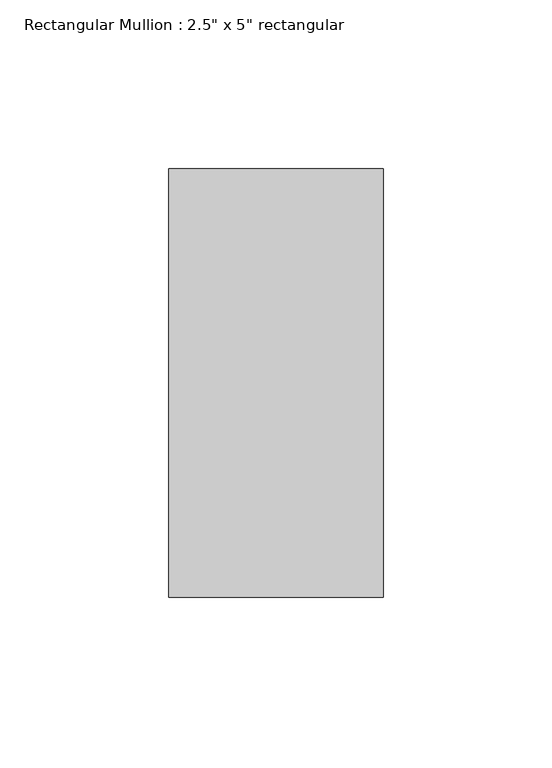
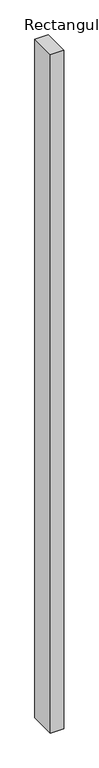
"""IFC4 building model written with IfcOpenShell, lengths in millimetres: member geometry."""

from ifc_helpers import new_model, si_unit, frame, origin, place, context, project, spatial, polyline, outline, extrude, source, transform, mapped, element, save


def member_6024fe87(model_context):
    return source(origin(), model_context, "Body", "SweptSolid", [
        extrude(outline(polyline([(0.0, 63.5), (0.0, -63.5), (-63.5, -63.5), (-63.5, 63.5), (0.0, 63.5)])), frame((0.0, 0.0, -3383.9874947), z_axis=(0.0, 0.0, 1.0), x_axis=(1.0, 0.0, 0.0)), (0.0, 0.0, 1.0), 3383.9874947),
    ])


if __name__ == "__main__":
    model = new_model("IFC4")
    model_context = context("Model", 3, world=origin())
    ifc_project = project(units=[si_unit("LENGTHUNIT", "METRE", prefix="MILLI")], contexts=[model_context])
    site = spatial("IfcSite", under=ifc_project)
    building = spatial("IfcBuilding", under=site)
    placement = place(None, origin())
    member_shape = member_6024fe87(model_context)
    element("IfcMember", 1, ObjectType="Rectangular Mullion : 2.5\" x 5\" rectangular", at=placement, inside=building, context=model_context, shape_type="MappedRepresentation", body=[
        mapped(member_shape, transform((0.0, 0.0, 0.0), x_axis=(1.0, 0.0, 0.0), y_axis=(0.0, 1.0, 0.0), z_axis=(0.0, 0.0, 1.0))),
    ])
    save(model, "model.ifc")

# Revit data of these elements
# Type "Rectangular Mullion : 2.5\" x 5\" rectangular"
#   built-in parameter 1007304 = 0.416667 (stored number, unit not read)
#   built-in parameter 1007301 = 0.104167 (stored number, unit not read)
#   built-in parameter 1007300 = 0.104167 (stored number, unit not read)
# Element 1 (IfcMember, "Rectangular Mullion : 2.5\" x 5\" rectangular")
#   Materials on its faces: "Aluminum"
# Materials
#   "Aluminum": class "Metal", colour RGB 247 247 247, transparency 0, Description = "Aluminum 6061", Cost = 0
